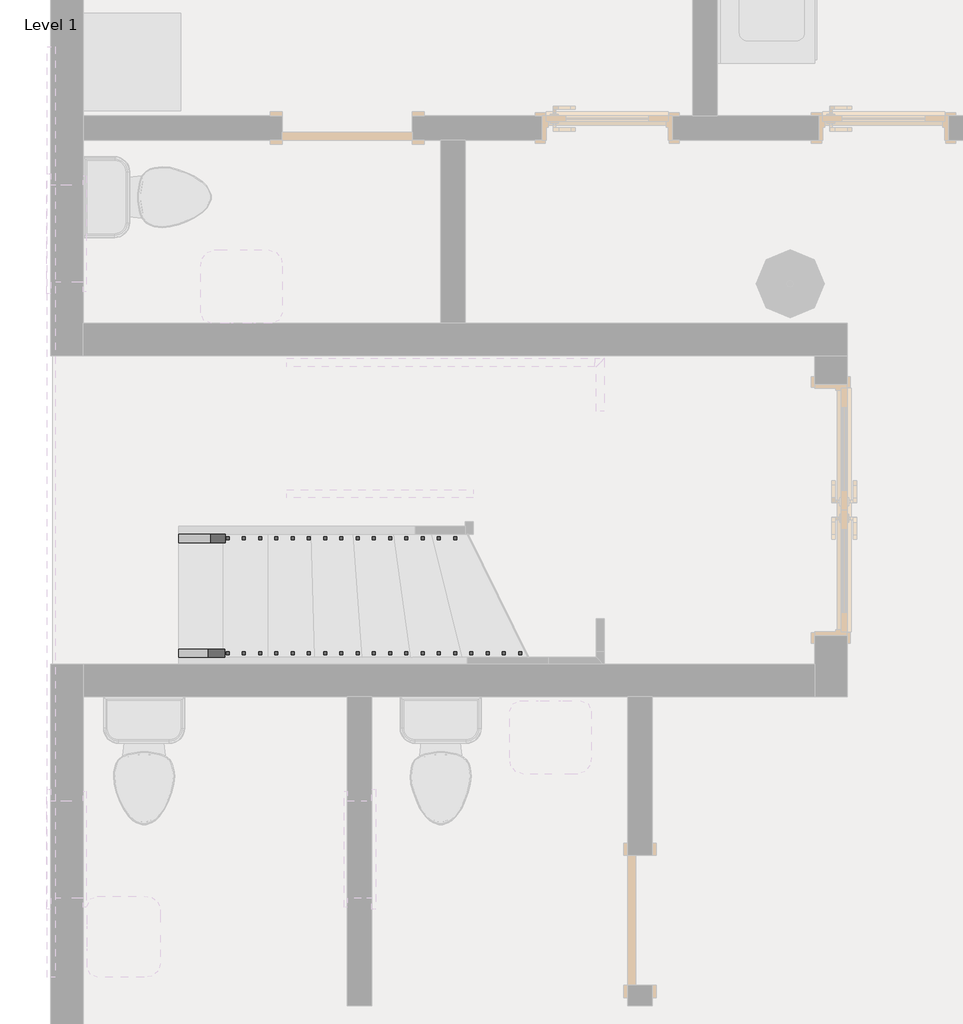
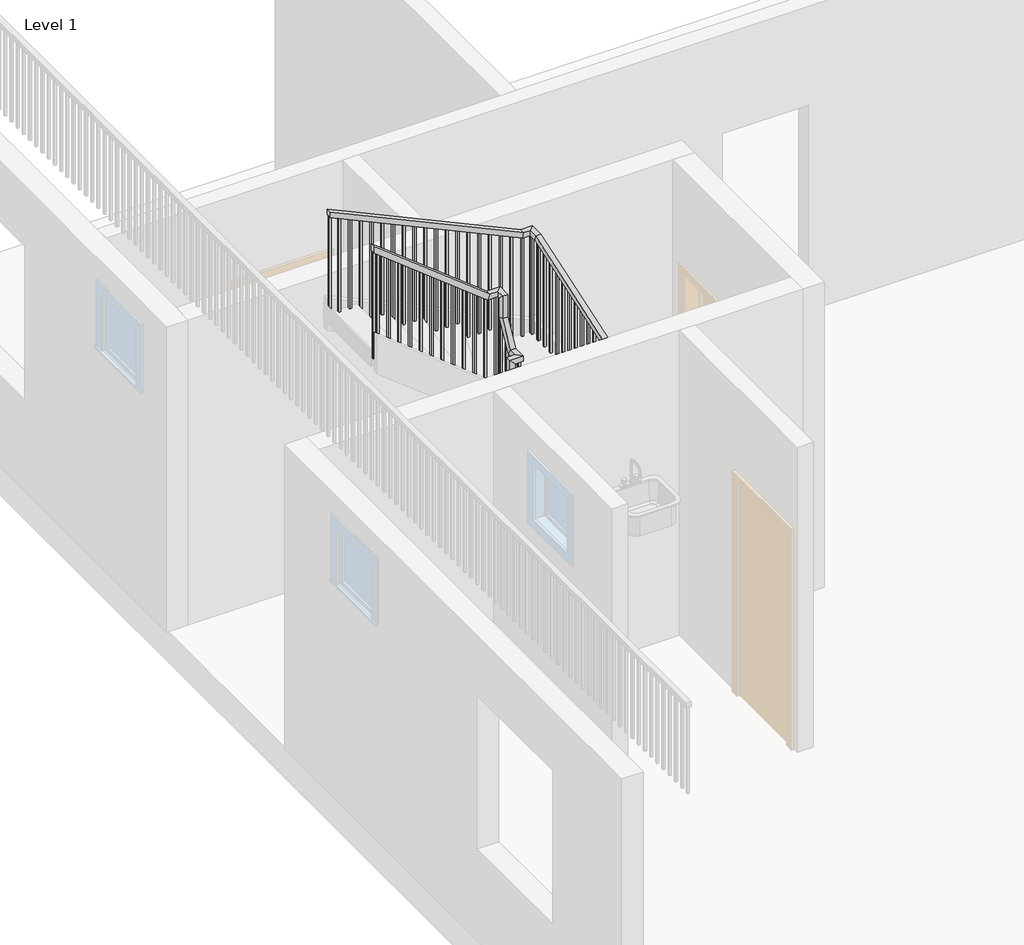
# One storey, part 4 of 7: 2 railings.
"""IFC4 building model written with IfcOpenShell, lengths in millimetres."""

from ifc_helpers import new_model, si_unit, frame, origin, place, context, project, spatial, polyline, outline, extrude, faceted_brep, element, save

model = new_model("IFC4")

# Units and contexts
model_context = context("Model", 3, world=origin())
ifc_project = project(units=[si_unit("LENGTHUNIT", "METRE", prefix="MILLI")], contexts=[model_context])

# Site, building, storey
site = spatial("IfcSite", under=ifc_project)
building = spatial("IfcBuilding", under=site)
storey = spatial("IfcBuildingStorey", under=building, Name="Level 1", Elevation=0.0)

# Railings
placement = place(None, origin())
element("IfcRailing", 1, ObjectType="Handrail - Rectangular", at=placement, inside=storey, context=model_context, shape_type="SolidModel", body=[
    faceted_brep([(-7679.0298583, 5229.7261204, 1101.5391642), (-7679.0298583, 5229.7261204, 1043.7493072), (-7679.0298583, 5178.9261204, 1043.7493072), (-7679.0298583, 5178.9261204, 1101.5391642), (-5235.2838113, 5229.7261204, 2426.8603355), (-5222.395286, 5229.7261204, 2376.0603355), (-5222.395286, 5178.9261204, 2376.0603355), (-5235.2838113, 5178.9261204, 2426.8603355), (-5120.1269231, 5229.7261204, 2376.0603355), (-5120.1269231, 5229.7261204, 2426.8603355), (-5120.1269231, 5429.9022511, 2426.8603355), (-5120.1269231, 5438.2536413, 2376.0603355), (-5069.3269231, 5178.9261204, 2376.0603355), (-5069.3269231, 5438.2536413, 2376.0603355), (-5069.3269231, 5178.9261204, 2426.8603355), (-5069.3269231, 5429.9022511, 2426.8603355), (-5120.1269231, 6946.2417743, 2857.587472), (-5120.1269231, 6946.2417743, 2908.387472), (-5180.0318978, 6946.2417743, 2908.387472), (-5191.2146936, 6946.2417743, 2857.587472), (-5069.3269231, 6997.0417743, 2857.587472), (-5191.2146936, 6997.0417743, 2857.587472), (-5069.3269231, 6997.0417743, 2908.387472), (-5180.0318978, 6997.0417743, 2908.387472), (-5120.1269231, 6854.8426939, 2908.387472), (-5120.1269231, 6863.1940841, 2857.587472), (-5069.3269231, 6863.1940841, 2857.587472), (-5069.3269231, 6854.8426939, 2908.387472), (-7005.4940547, 6946.2417743, 3753.0086233), (-7005.4940547, 6997.0417743, 3753.0086233), (-7005.4940547, 6997.0417743, 3697.0344673), (-7005.4940547, 6946.2417743, 3697.0344673)], [[[0, 1, 2, 3]], [[1, 0, 4, 5]], [[2, 1, 5, 6]], [[3, 2, 6, 7]], [[0, 3, 7, 4]], [[8, 9, 10, 11]], [[12, 8, 11, 13]], [[14, 12, 13, 15]], [[9, 14, 15, 10]], [[16, 17, 18, 19]], [[20, 16, 19, 21]], [[22, 20, 21, 23]], [[17, 22, 23, 18]], [[5, 4, 9, 8]], [[6, 5, 8, 12]], [[7, 6, 12, 14]], [[4, 7, 14, 9]], [[11, 10, 24, 25]], [[13, 11, 25, 26]], [[15, 13, 26, 27]], [[10, 15, 27, 24]], [[25, 24, 17, 16]], [[26, 25, 16, 20]], [[27, 26, 20, 22]], [[24, 27, 22, 17]], [[28, 29, 30, 31]], [[19, 18, 28, 31]], [[21, 19, 31, 30]], [[23, 21, 30, 29]], [[18, 23, 29, 28]]]),
    extrude(outline(polyline([(3647.1625419, -6897.7068978), (3655.9767662, -6916.7568978), (2709.3333333, -6916.7568978), (2709.3333333, -6897.7068978), (3647.1625419, -6897.7068978)])), frame((0.0, 6962.1167743, 0.0), z_axis=(0.0, 1.0, 0.0), x_axis=(0.0, 0.0, 1.0)), (0.0, 0.0, 1.0), 19.05),
    extrude(outline(polyline([(3600.1533456, -6796.1068978), (3608.9675699, -6815.1568978), (2709.3333333, -6815.1568978), (2709.3333333, -6796.1068978), (3600.1533456, -6796.1068978)])), frame((0.0, 6962.1167743, 0.0), z_axis=(0.0, 1.0, 0.0), x_axis=(0.0, 0.0, 1.0)), (0.0, 0.0, 1.0), 19.05),
    extrude(outline(polyline([(3553.1441492, -6694.5068978), (3561.9583735, -6713.5568978), (2540.0, -6713.5568978), (2540.0, -6694.5068978), (3553.1441492, -6694.5068978)])), frame((0.0, 6962.1167743, 0.0), z_axis=(0.0, 1.0, 0.0), x_axis=(0.0, 0.0, 1.0)), (0.0, 0.0, 1.0), 19.05),
    extrude(outline(polyline([(3506.1349529, -6592.9068978), (3514.9491772, -6611.9568978), (2540.0, -6611.9568978), (2540.0, -6592.9068978), (3506.1349529, -6592.9068978)])), frame((0.0, 6962.1167743, 0.0), z_axis=(0.0, 1.0, 0.0), x_axis=(0.0, 0.0, 1.0)), (0.0, 0.0, 1.0), 19.05),
    extrude(outline(polyline([(3459.1257565, -6491.3068978), (3467.9399808, -6510.3568978), (2540.0, -6510.3568978), (2540.0, -6491.3068978), (3459.1257565, -6491.3068978)])), frame((0.0, 6962.1167743, 0.0), z_axis=(0.0, 1.0, 0.0), x_axis=(0.0, 0.0, 1.0)), (0.0, 0.0, 1.0), 19.05),
    extrude(outline(polyline([(3412.1165601, -6389.7068978), (3420.9307845, -6408.7568978), (2370.6666667, -6408.7568978), (2370.6666667, -6389.7068978), (3412.1165601, -6389.7068978)])), frame((0.0, 6962.1167743, 0.0), z_axis=(0.0, 1.0, 0.0), x_axis=(0.0, 0.0, 1.0)), (0.0, 0.0, 1.0), 19.05),
    extrude(outline(polyline([(3365.1073638, -6288.1068978), (3373.9215881, -6307.1568978), (2370.6666667, -6307.1568978), (2370.6666667, -6288.1068978), (3365.1073638, -6288.1068978)])), frame((0.0, 6962.1167743, 0.0), z_axis=(0.0, 1.0, 0.0), x_axis=(0.0, 0.0, 1.0)), (0.0, 0.0, 1.0), 19.05),
    extrude(outline(polyline([(3318.0981674, -6186.5068978), (3326.9123918, -6205.5568978), (2370.6666667, -6205.5568978), (2370.6666667, -6186.5068978), (3318.0981674, -6186.5068978)])), frame((0.0, 6962.1167743, 0.0), z_axis=(0.0, 1.0, 0.0), x_axis=(0.0, 0.0, 1.0)), (0.0, 0.0, 1.0), 19.05),
    extrude(outline(polyline([(3271.0889711, -6084.9068978), (3279.9031954, -6103.9568978), (2201.3333333, -6103.9568978), (2201.3333333, -6084.9068978), (3271.0889711, -6084.9068978)])), frame((0.0, 6962.1167743, 0.0), z_axis=(0.0, 1.0, 0.0), x_axis=(0.0, 0.0, 1.0)), (0.0, 0.0, 1.0), 19.05),
    extrude(outline(polyline([(3224.0797747, -5983.3068978), (3232.8939991, -6002.3568978), (2201.3333333, -6002.3568978), (2201.3333333, -5983.3068978), (3224.0797747, -5983.3068978)])), frame((0.0, 6962.1167743, 0.0), z_axis=(0.0, 1.0, 0.0), x_axis=(0.0, 0.0, 1.0)), (0.0, 0.0, 1.0), 19.05),
    extrude(outline(polyline([(3177.0705784, -5881.7068978), (3185.8848027, -5900.7568978), (2201.3333333, -5900.7568978), (2201.3333333, -5881.7068978), (3177.0705784, -5881.7068978)])), frame((0.0, 6962.1167743, 0.0), z_axis=(0.0, 1.0, 0.0), x_axis=(0.0, 0.0, 1.0)), (0.0, 0.0, 1.0), 19.05),
    extrude(outline(polyline([(3130.061382, -5780.1068978), (3138.8756063, -5799.1568978), (2201.3333333, -5799.1568978), (2201.3333333, -5780.1068978), (3130.061382, -5780.1068978)])), frame((0.0, 6962.1167743, 0.0), z_axis=(0.0, 1.0, 0.0), x_axis=(0.0, 0.0, 1.0)), (0.0, 0.0, 1.0), 19.05),
    extrude(outline(polyline([(3083.0521857, -5678.5068978), (3091.86641, -5697.5568978), (2032.0, -5697.5568978), (2032.0, -5678.5068978), (3083.0521857, -5678.5068978)])), frame((0.0, 6962.1167743, 0.0), z_axis=(0.0, 1.0, 0.0), x_axis=(0.0, 0.0, 1.0)), (0.0, 0.0, 1.0), 19.05),
    extrude(outline(polyline([(3036.0429893, -5576.9068978), (3044.8572136, -5595.9568978), (2032.0, -5595.9568978), (2032.0, -5576.9068978), (3036.0429893, -5576.9068978)])), frame((0.0, 6962.1167743, 0.0), z_axis=(0.0, 1.0, 0.0), x_axis=(0.0, 0.0, 1.0)), (0.0, 0.0, 1.0), 19.05),
    extrude(outline(polyline([(2989.033793, -5475.3068978), (2997.8480173, -5494.3568978), (2032.0, -5494.3568978), (2032.0, -5475.3068978), (2989.033793, -5475.3068978)])), frame((0.0, 6962.1167743, 0.0), z_axis=(0.0, 1.0, 0.0), x_axis=(0.0, 0.0, 1.0)), (0.0, 0.0, 1.0), 19.05),
    extrude(outline(polyline([(2942.0245966, -5373.7068978), (2950.8388209, -5392.7568978), (2032.0, -5392.7568978), (2032.0, -5373.7068978), (2942.0245966, -5373.7068978)])), frame((0.0, 6962.1167743, 0.0), z_axis=(0.0, 1.0, 0.0), x_axis=(0.0, 0.0, 1.0)), (0.0, 0.0, 1.0), 19.05),
    extrude(outline(polyline([(2895.0154003, -5272.1068978), (2903.8296246, -5291.1568978), (1862.6666667, -5291.1568978), (1862.6666667, -5272.1068978), (2895.0154003, -5272.1068978)])), frame((0.0, 6962.1167743, 0.0), z_axis=(0.0, 1.0, 0.0), x_axis=(0.0, 0.0, 1.0)), (0.0, 0.0, 1.0), 19.05),
    extrude(outline(polyline([(-5085.2019231, 6946.9176939), (-5104.2519231, 6946.9176939), (-5104.2519231, 6965.9676939), (-5085.2019231, 6965.9676939), (-5085.2019231, 6946.9176939)])), frame((0.0, 0.0, 1862.6666667), z_axis=(0.0, 0.0, 1.0), x_axis=(1.0, 0.0, 0.0)), (0.0, 0.0, 1.0), 994.9208054),
    extrude(outline(polyline([(6842.7772511, 2850.6880545), (6861.8272511, 2857.125581), (6861.8272511, 1862.6666667), (6842.7772511, 1862.6666667), (6842.7772511, 2850.6880545)])), frame((-5104.2519231, 0.0, 0.0), z_axis=(1.0, 0.0, 0.0), x_axis=(0.0, 1.0, 0.0)), (0.0, 0.0, 1.0), 19.05),
    extrude(outline(polyline([(6741.1772511, 2816.3545795), (6760.2272511, 2822.792106), (6760.2272511, 1862.6666667), (6741.1772511, 1862.6666667), (6741.1772511, 2816.3545795)])), frame((-5104.2519231, 0.0, 0.0), z_axis=(1.0, 0.0, 0.0), x_axis=(0.0, 1.0, 0.0)), (0.0, 0.0, 1.0), 19.05),
    extrude(outline(polyline([(6639.5772511, 2782.0211045), (6658.6272511, 2788.458631), (6658.6272511, 1862.6666667), (6639.5772511, 1862.6666667), (6639.5772511, 2782.0211045)])), frame((-5104.2519231, 0.0, 0.0), z_axis=(1.0, 0.0, 0.0), x_axis=(0.0, 1.0, 0.0)), (0.0, 0.0, 1.0), 19.05),
    extrude(outline(polyline([(6537.9772511, 2747.6876295), (6557.0272511, 2754.125156), (6557.0272511, 1862.6666667), (6537.9772511, 1862.6666667), (6537.9772511, 2747.6876295)])), frame((-5104.2519231, 0.0, 0.0), z_axis=(1.0, 0.0, 0.0), x_axis=(0.0, 1.0, 0.0)), (0.0, 0.0, 1.0), 19.05),
    extrude(outline(polyline([(6436.3772511, 2713.3541545), (6455.4272511, 2719.791681), (6455.4272511, 1693.3333333), (6436.3772511, 1693.3333333), (6436.3772511, 2713.3541545)])), frame((-5104.2519231, 0.0, 0.0), z_axis=(1.0, 0.0, 0.0), x_axis=(0.0, 1.0, 0.0)), (0.0, 0.0, 1.0), 19.05),
    extrude(outline(polyline([(6334.7772511, 2679.0206795), (6353.8272511, 2685.458206), (6353.8272511, 1693.3333333), (6334.7772511, 1693.3333333), (6334.7772511, 2679.0206795)])), frame((-5104.2519231, 0.0, 0.0), z_axis=(1.0, 0.0, 0.0), x_axis=(0.0, 1.0, 0.0)), (0.0, 0.0, 1.0), 19.05),
    extrude(outline(polyline([(6233.1772511, 2644.6872045), (6252.2272511, 2651.124731), (6252.2272511, 1693.3333333), (6233.1772511, 1693.3333333), (6233.1772511, 2644.6872045)])), frame((-5104.2519231, 0.0, 0.0), z_axis=(1.0, 0.0, 0.0), x_axis=(0.0, 1.0, 0.0)), (0.0, 0.0, 1.0), 19.05),
    extrude(outline(polyline([(6131.5772511, 2610.3537294), (6150.6272511, 2616.791256), (6150.6272511, 1693.3333333), (6131.5772511, 1693.3333333), (6131.5772511, 2610.3537294)])), frame((-5104.2519231, 0.0, 0.0), z_axis=(1.0, 0.0, 0.0), x_axis=(0.0, 1.0, 0.0)), (0.0, 0.0, 1.0), 19.05),
    extrude(outline(polyline([(6029.9772511, 2576.0202544), (6049.0272511, 2582.457781), (6049.0272511, 1693.3333333), (6029.9772511, 1693.3333333), (6029.9772511, 2576.0202544)])), frame((-5104.2519231, 0.0, 0.0), z_axis=(1.0, 0.0, 0.0), x_axis=(0.0, 1.0, 0.0)), (0.0, 0.0, 1.0), 19.05),
    extrude(outline(polyline([(5928.3772511, 2541.6867794), (5947.4272511, 2548.124306), (5947.4272511, 1524.0), (5928.3772511, 1524.0), (5928.3772511, 2541.6867794)])), frame((-5104.2519231, 0.0, 0.0), z_axis=(1.0, 0.0, 0.0), x_axis=(0.0, 1.0, 0.0)), (0.0, 0.0, 1.0), 19.05),
    extrude(outline(polyline([(5826.7772511, 2507.3533044), (5845.8272511, 2513.790831), (5845.8272511, 1524.0), (5826.7772511, 1524.0), (5826.7772511, 2507.3533044)])), frame((-5104.2519231, 0.0, 0.0), z_axis=(1.0, 0.0, 0.0), x_axis=(0.0, 1.0, 0.0)), (0.0, 0.0, 1.0), 19.05),
    extrude(outline(polyline([(5725.1772511, 2473.0198294), (5744.2272511, 2479.457356), (5744.2272511, 1524.0), (5725.1772511, 1524.0), (5725.1772511, 2473.0198294)])), frame((-5104.2519231, 0.0, 0.0), z_axis=(1.0, 0.0, 0.0), x_axis=(0.0, 1.0, 0.0)), (0.0, 0.0, 1.0), 19.05),
    extrude(outline(polyline([(5623.5772511, 2438.6863544), (5642.6272511, 2445.123881), (5642.6272511, 1524.0), (5623.5772511, 1524.0), (5623.5772511, 2438.6863544)])), frame((-5104.2519231, 0.0, 0.0), z_axis=(1.0, 0.0, 0.0), x_axis=(0.0, 1.0, 0.0)), (0.0, 0.0, 1.0), 19.05),
    extrude(outline(polyline([(5521.9772511, 2404.3528794), (5541.0272511, 2410.790406), (5541.0272511, 1524.0), (5521.9772511, 1524.0), (5521.9772511, 2404.3528794)])), frame((-5104.2519231, 0.0, 0.0), z_axis=(1.0, 0.0, 0.0), x_axis=(0.0, 1.0, 0.0)), (0.0, 0.0, 1.0), 19.05),
    extrude(outline(polyline([(-5085.2019231, 5398.0011204), (-5104.2519231, 5398.0011204), (-5104.2519231, 5417.0511204), (-5085.2019231, 5417.0511204), (-5085.2019231, 5398.0011204)])), frame((0.0, 0.0, 1354.6666667), z_axis=(0.0, 0.0, 1.0), x_axis=(1.0, 0.0, 0.0)), (0.0, 0.0, 1.0), 1021.3936688),
    extrude(outline(polyline([(-5085.2019231, 5296.4011204), (-5104.2519231, 5296.4011204), (-5104.2519231, 5315.4511204), (-5085.2019231, 5315.4511204), (-5085.2019231, 5296.4011204)])), frame((0.0, 0.0, 1354.6666667), z_axis=(0.0, 0.0, 1.0), x_axis=(1.0, 0.0, 0.0)), (0.0, 0.0, 1.0), 1021.3936688),
    extrude(outline(polyline([(-5143.2088113, 5194.8011204), (-5143.2088113, 5213.8511204), (-5124.1588113, 5213.8511204), (-5124.1588113, 5194.8011204), (-5143.2088113, 5194.8011204)])), frame((0.0, 0.0, 1354.6666667), z_axis=(0.0, 0.0, 1.0), x_axis=(1.0, 0.0, 0.0)), (0.0, 0.0, 1.0), 1021.3936688),
    extrude(outline(polyline([(2371.3368575, -5231.1048583), (2361.0054369, -5250.1548583), (1354.6666667, -5250.1548583), (1354.6666667, -5231.1048583), (2371.3368575, -5231.1048583)])), frame((0.0, 5194.8011204, 0.0), z_axis=(0.0, 1.0, 0.0), x_axis=(0.0, 0.0, 1.0)), (0.0, 0.0, 1.0), 19.05),
    extrude(outline(polyline([(2316.2359475, -5332.7048583), (2305.9045269, -5351.7548583), (1354.6666667, -5351.7548583), (1354.6666667, -5332.7048583), (2316.2359475, -5332.7048583)])), frame((0.0, 5194.8011204, 0.0), z_axis=(0.0, 1.0, 0.0), x_axis=(0.0, 0.0, 1.0)), (0.0, 0.0, 1.0), 19.05),
    extrude(outline(polyline([(2261.1350375, -5434.3048583), (2250.8036169, -5453.3548583), (1354.6666667, -5453.3548583), (1354.6666667, -5434.3048583), (2261.1350375, -5434.3048583)])), frame((0.0, 5194.8011204, 0.0), z_axis=(0.0, 1.0, 0.0), x_axis=(0.0, 0.0, 1.0)), (0.0, 0.0, 1.0), 19.05),
    extrude(outline(polyline([(2206.0341275, -5535.9048583), (2195.7027069, -5554.9548583), (1185.3333333, -5554.9548583), (1185.3333333, -5535.9048583), (2206.0341275, -5535.9048583)])), frame((0.0, 5194.8011204, 0.0), z_axis=(0.0, 1.0, 0.0), x_axis=(0.0, 0.0, 1.0)), (0.0, 0.0, 1.0), 19.05),
    extrude(outline(polyline([(2150.9332175, -5637.5048583), (2140.6017969, -5656.5548583), (1185.3333333, -5656.5548583), (1185.3333333, -5637.5048583), (2150.9332175, -5637.5048583)])), frame((0.0, 5194.8011204, 0.0), z_axis=(0.0, 1.0, 0.0), x_axis=(0.0, 0.0, 1.0)), (0.0, 0.0, 1.0), 19.05),
    extrude(outline(polyline([(2095.8323075, -5739.1048583), (2085.5008869, -5758.1548583), (1185.3333333, -5758.1548583), (1185.3333333, -5739.1048583), (2095.8323075, -5739.1048583)])), frame((0.0, 5194.8011204, 0.0), z_axis=(0.0, 1.0, 0.0), x_axis=(0.0, 0.0, 1.0)), (0.0, 0.0, 1.0), 19.05),
    extrude(outline(polyline([(2040.7313975, -5840.7048583), (2030.3999769, -5859.7548583), (1185.3333333, -5859.7548583), (1185.3333333, -5840.7048583), (2040.7313975, -5840.7048583)])), frame((0.0, 5194.8011204, 0.0), z_axis=(0.0, 1.0, 0.0), x_axis=(0.0, 0.0, 1.0)), (0.0, 0.0, 1.0), 19.05),
    extrude(outline(polyline([(1985.6304875, -5942.3048583), (1975.2990669, -5961.3548583), (1016.0, -5961.3548583), (1016.0, -5942.3048583), (1985.6304875, -5942.3048583)])), frame((0.0, 5194.8011204, 0.0), z_axis=(0.0, 1.0, 0.0), x_axis=(0.0, 0.0, 1.0)), (0.0, 0.0, 1.0), 19.05),
    extrude(outline(polyline([(1930.5295775, -6043.9048583), (1920.1981569, -6062.9548583), (1016.0, -6062.9548583), (1016.0, -6043.9048583), (1930.5295775, -6043.9048583)])), frame((0.0, 5194.8011204, 0.0), z_axis=(0.0, 1.0, 0.0), x_axis=(0.0, 0.0, 1.0)), (0.0, 0.0, 1.0), 19.05),
    extrude(outline(polyline([(1875.4286675, -6145.5048583), (1865.0972469, -6164.5548583), (1016.0, -6164.5548583), (1016.0, -6145.5048583), (1875.4286675, -6145.5048583)])), frame((0.0, 5194.8011204, 0.0), z_axis=(0.0, 1.0, 0.0), x_axis=(0.0, 0.0, 1.0)), (0.0, 0.0, 1.0), 19.05),
    extrude(outline(polyline([(1820.3277575, -6247.1048583), (1809.9963369, -6266.1548583), (846.6666667, -6266.1548583), (846.6666667, -6247.1048583), (1820.3277575, -6247.1048583)])), frame((0.0, 5194.8011204, 0.0), z_axis=(0.0, 1.0, 0.0), x_axis=(0.0, 0.0, 1.0)), (0.0, 0.0, 1.0), 19.05),
    extrude(outline(polyline([(1765.2268475, -6348.7048583), (1754.8954269, -6367.7548583), (846.6666667, -6367.7548583), (846.6666667, -6348.7048583), (1765.2268475, -6348.7048583)])), frame((0.0, 5194.8011204, 0.0), z_axis=(0.0, 1.0, 0.0), x_axis=(0.0, 0.0, 1.0)), (0.0, 0.0, 1.0), 19.05),
    extrude(outline(polyline([(1710.1259375, -6450.3048583), (1699.7945169, -6469.3548583), (846.6666667, -6469.3548583), (846.6666667, -6450.3048583), (1710.1259375, -6450.3048583)])), frame((0.0, 5194.8011204, 0.0), z_axis=(0.0, 1.0, 0.0), x_axis=(0.0, 0.0, 1.0)), (0.0, 0.0, 1.0), 19.05),
    extrude(outline(polyline([(1655.0250275, -6551.9048583), (1644.6936069, -6570.9548583), (677.3333333, -6570.9548583), (677.3333333, -6551.9048583), (1655.0250275, -6551.9048583)])), frame((0.0, 5194.8011204, 0.0), z_axis=(0.0, 1.0, 0.0), x_axis=(0.0, 0.0, 1.0)), (0.0, 0.0, 1.0), 19.05),
    extrude(outline(polyline([(1599.9241175, -6653.5048583), (1589.5926969, -6672.5548583), (677.3333333, -6672.5548583), (677.3333333, -6653.5048583), (1599.9241175, -6653.5048583)])), frame((0.0, 5194.8011204, 0.0), z_axis=(0.0, 1.0, 0.0), x_axis=(0.0, 0.0, 1.0)), (0.0, 0.0, 1.0), 19.05),
    extrude(outline(polyline([(1544.8232075, -6755.1048583), (1534.4917869, -6774.1548583), (677.3333333, -6774.1548583), (677.3333333, -6755.1048583), (1544.8232075, -6755.1048583)])), frame((0.0, 5194.8011204, 0.0), z_axis=(0.0, 1.0, 0.0), x_axis=(0.0, 0.0, 1.0)), (0.0, 0.0, 1.0), 19.05),
    extrude(outline(polyline([(1489.7222975, -6856.7048583), (1479.3908769, -6875.7548583), (508.0, -6875.7548583), (508.0, -6856.7048583), (1489.7222975, -6856.7048583)])), frame((0.0, 5194.8011204, 0.0), z_axis=(0.0, 1.0, 0.0), x_axis=(0.0, 0.0, 1.0)), (0.0, 0.0, 1.0), 19.05),
    extrude(outline(polyline([(1434.6213875, -6958.3048583), (1424.2899669, -6977.3548583), (508.0, -6977.3548583), (508.0, -6958.3048583), (1434.6213875, -6958.3048583)])), frame((0.0, 5194.8011204, 0.0), z_axis=(0.0, 1.0, 0.0), x_axis=(0.0, 0.0, 1.0)), (0.0, 0.0, 1.0), 19.05),
    extrude(outline(polyline([(1379.5204775, -7059.9048583), (1369.1890569, -7078.9548583), (508.0, -7078.9548583), (508.0, -7059.9048583), (1379.5204775, -7059.9048583)])), frame((0.0, 5194.8011204, 0.0), z_axis=(0.0, 1.0, 0.0), x_axis=(0.0, 0.0, 1.0)), (0.0, 0.0, 1.0), 19.05),
    extrude(outline(polyline([(1324.4195675, -7161.5048583), (1314.0881469, -7180.5548583), (338.6666667, -7180.5548583), (338.6666667, -7161.5048583), (1324.4195675, -7161.5048583)])), frame((0.0, 5194.8011204, 0.0), z_axis=(0.0, 1.0, 0.0), x_axis=(0.0, 0.0, 1.0)), (0.0, 0.0, 1.0), 19.05),
    extrude(outline(polyline([(1269.3186575, -7263.1048583), (1258.9872369, -7282.1548583), (338.6666667, -7282.1548583), (338.6666667, -7263.1048583), (1269.3186575, -7263.1048583)])), frame((0.0, 5194.8011204, 0.0), z_axis=(0.0, 1.0, 0.0), x_axis=(0.0, 0.0, 1.0)), (0.0, 0.0, 1.0), 19.05),
    extrude(outline(polyline([(1214.2177475, -7364.7048583), (1203.8863269, -7383.7548583), (338.6666667, -7383.7548583), (338.6666667, -7364.7048583), (1214.2177475, -7364.7048583)])), frame((0.0, 5194.8011204, 0.0), z_axis=(0.0, 1.0, 0.0), x_axis=(0.0, 0.0, 1.0)), (0.0, 0.0, 1.0), 19.05),
    extrude(outline(polyline([(1159.1168375, -7466.3048583), (1148.7854169, -7485.3548583), (169.3333333, -7485.3548583), (169.3333333, -7466.3048583), (1159.1168375, -7466.3048583)])), frame((0.0, 5194.8011204, 0.0), z_axis=(0.0, 1.0, 0.0), x_axis=(0.0, 0.0, 1.0)), (0.0, 0.0, 1.0), 19.05),
    extrude(outline(polyline([(1104.0159275, -7567.9048583), (1093.6845069, -7586.9548583), (169.3333333, -7586.9548583), (169.3333333, -7567.9048583), (1104.0159275, -7567.9048583)])), frame((0.0, 5194.8011204, 0.0), z_axis=(0.0, 1.0, 0.0), x_axis=(0.0, 0.0, 1.0)), (0.0, 0.0, 1.0), 19.05),
    extrude(outline(polyline([(-5170.5068978, 6981.1667743), (-5170.5068978, 6962.1167743), (-5189.5568978, 6962.1167743), (-5189.5568978, 6981.1667743), (-5170.5068978, 6981.1667743)])), frame((0.0, 0.0, 1862.6666667), z_axis=(0.0, 0.0, 1.0), x_axis=(1.0, 0.0, 0.0)), (0.0, 0.0, 1.0), 994.9208054),
    extrude(outline(polyline([(-5085.2019231, 6962.1167743), (-5104.2519231, 6962.1167743), (-5104.2519231, 6981.1667743), (-5085.2019231, 6981.1667743), (-5085.2019231, 6962.1167743)])), frame((0.0, 0.0, 1862.6666667), z_axis=(0.0, 0.0, 1.0), x_axis=(1.0, 0.0, 0.0)), (0.0, 0.0, 1.0), 994.9208054),
    extrude(outline(polyline([(6845.3176939, 2851.546541), (6864.3676939, 2857.9840675), (6864.3676939, 1862.6666667), (6845.3176939, 1862.6666667), (6845.3176939, 2851.546541)])), frame((-5104.2519231, 0.0, 0.0), z_axis=(1.0, 0.0, 0.0), x_axis=(0.0, 1.0, 0.0)), (0.0, 0.0, 1.0), 19.05),
    extrude(outline(polyline([(-5085.2019231, 5420.3772511), (-5104.2519231, 5420.3772511), (-5104.2519231, 5439.4272511), (-5085.2019231, 5439.4272511), (-5085.2019231, 5420.3772511)])), frame((0.0, 0.0, 1354.6666667), z_axis=(0.0, 0.0, 1.0), x_axis=(1.0, 0.0, 0.0)), (0.0, 0.0, 1.0), 1021.3936688),
    extrude(outline(polyline([(-5104.2519231, 5194.8011204), (-5104.2519231, 5213.8511204), (-5085.2019231, 5213.8511204), (-5085.2019231, 5194.8011204), (-5104.2519231, 5194.8011204)])), frame((0.0, 0.0, 1354.6666667), z_axis=(0.0, 0.0, 1.0), x_axis=(1.0, 0.0, 0.0)), (0.0, 0.0, 1.0), 1021.3936688),
    extrude(outline(polyline([(2374.2361888, -5225.7588113), (2363.9047682, -5244.8088113), (1354.6666667, -5244.8088113), (1354.6666667, -5225.7588113), (2374.2361888, -5225.7588113)])), frame((0.0, 5194.8011204, 0.0), z_axis=(0.0, 1.0, 0.0), x_axis=(0.0, 0.0, 1.0)), (0.0, 0.0, 1.0), 19.05),
    extrude(outline(polyline([(3688.220243, -6986.4440547), (3697.0344673, -7005.4940547), (2709.3333333, -7005.4940547), (2709.3333333, -6986.4440547), (3688.220243, -6986.4440547)])), frame((0.0, 6962.1167743, 0.0), z_axis=(0.0, 1.0, 0.0), x_axis=(0.0, 0.0, 1.0)), (0.0, 0.0, 1.0), 19.05),
    extrude(outline(polyline([(1054.0807278, -7659.9798583), (1043.7493072, -7679.0298583), (169.3333333, -7679.0298583), (169.3333333, -7659.9798583), (1054.0807278, -7659.9798583)])), frame((0.0, 5194.8011204, 0.0), z_axis=(0.0, 1.0, 0.0), x_axis=(0.0, 0.0, 1.0)), (0.0, 0.0, 1.0), 19.05),
])
element("IfcRailing", 2, ObjectType="Handrail - Rectangular", at=placement, inside=storey, context=model_context, shape_type="SolidModel", body=[
    faceted_brep([(-7679.0298583, 5948.2839473, 1063.2569244), (-7679.0298583, 5948.2839473, 1001.8432483), (-7679.0298583, 5897.4839473, 1001.8432483), (-7679.0298583, 5897.4839473, 1063.2569244), (-5914.88475, 5948.2839473, 2261.724814), (-5864.08475, 5948.2839473, 2234.8220001), (-5864.08475, 5897.4839473, 2234.8220001), (-5914.88475, 5897.4839473, 2261.724814), (-5838.68475, 6054.8875761, 2473.5239648), (-5838.68475, 6024.4839473, 2524.3239648), (-5838.68475, 6151.4839473, 2761.1854815), (-5838.68475, 6202.2839473, 2748.4257604), (-5787.88475, 6054.8875761, 2473.5239648), (-5787.88475, 6202.2839473, 2748.4257604), (-5787.88475, 6024.4839473, 2524.3239648), (-5787.88475, 6151.4839473, 2761.1854815), (-7005.4940547, 6227.6839473, 3843.0590007), (-7005.4940547, 6278.4839473, 3843.0590007), (-7005.4940547, 6278.4839473, 3778.4769091), (-7005.4940547, 6227.6839473, 3778.4769091), (-5932.4418214, 6227.6839473, 2936.143705), (-5914.88475, 6227.6839473, 2986.943705), (-5932.4418214, 6278.4839473, 2936.143705), (-5914.88475, 6278.4839473, 2986.943705), (-5914.88475, 5948.2839473, 2524.3239648), (-5864.08475, 5948.2839473, 2473.5239648), (-5864.08475, 5897.4839473, 2473.5239648), (-5914.88475, 5897.4839473, 2524.3239648), (-5838.68475, 5948.2839473, 2524.3239648), (-5838.68475, 5948.2839473, 2473.5239648), (-5787.88475, 5897.4839473, 2473.5239648), (-5787.88475, 5897.4839473, 2524.3239648), (-5838.68475, 6151.4839473, 2986.943705), (-5838.68475, 6202.2839473, 2936.143705), (-5787.88475, 6202.2839473, 2936.143705), (-5787.88475, 6151.4839473, 2986.943705), (-5838.68475, 6227.6839473, 2986.943705), (-5838.68475, 6227.6839473, 2936.143705), (-5787.88475, 6278.4839473, 2936.143705), (-5787.88475, 6278.4839473, 2986.943705)], [[[0, 1, 2, 3]], [[1, 0, 4, 5]], [[2, 1, 5, 6]], [[3, 2, 6, 7]], [[0, 3, 7, 4]], [[8, 9, 10, 11]], [[12, 8, 11, 13]], [[14, 12, 13, 15]], [[9, 14, 15, 10]], [[16, 17, 18, 19]], [[20, 21, 16, 19]], [[22, 20, 19, 18]], [[23, 22, 18, 17]], [[21, 23, 17, 16]], [[5, 4, 24, 25]], [[6, 5, 25, 26]], [[7, 6, 26, 27]], [[4, 7, 27, 24]], [[25, 24, 28, 29]], [[26, 25, 29, 30]], [[27, 26, 30, 31]], [[24, 27, 31, 28]], [[29, 28, 9, 8]], [[30, 29, 8, 12]], [[31, 30, 12, 14]], [[28, 31, 14, 9]], [[11, 10, 32, 33]], [[13, 11, 33, 34]], [[15, 13, 34, 35]], [[10, 15, 35, 32]], [[33, 32, 36, 37]], [[34, 33, 37, 38]], [[35, 34, 38, 39]], [[32, 35, 39, 36]], [[37, 36, 21, 20]], [[38, 37, 20, 22]], [[39, 38, 22, 23]], [[36, 39, 23, 21]]]),
    extrude(outline(polyline([(3749.1293953, -6968.1081187), (2709.3333333, -6968.1081187), (2709.3333333, -6949.0581187), (3734.1753725, -6949.0581187), (3749.1293953, -6968.1081187)])), frame((0.0, 6243.5589473, 0.0), z_axis=(0.0, 1.0, 0.0), x_axis=(0.0, 0.0, 1.0)), (0.0, 0.0, 1.0), 19.05),
    extrude(outline(polyline([(3669.3746071, -6866.5081187), (2709.3333333, -6866.5081187), (2709.3333333, -6847.4581187), (3654.4205844, -6847.4581187), (3669.3746071, -6866.5081187)])), frame((0.0, 6243.5589473, 0.0), z_axis=(0.0, 1.0, 0.0), x_axis=(0.0, 0.0, 1.0)), (0.0, 0.0, 1.0), 19.05),
    extrude(outline(polyline([(3589.619819, -6764.9081187), (2709.3333333, -6764.9081187), (2709.3333333, -6745.8581187), (3574.6657962, -6745.8581187), (3589.619819, -6764.9081187)])), frame((0.0, 6243.5589473, 0.0), z_axis=(0.0, 1.0, 0.0), x_axis=(0.0, 0.0, 1.0)), (0.0, 0.0, 1.0), 19.05),
    extrude(outline(polyline([(3509.8650309, -6663.3081187), (2540.0, -6663.3081187), (2540.0, -6644.2581187), (3494.9110081, -6644.2581187), (3509.8650309, -6663.3081187)])), frame((0.0, 6243.5589473, 0.0), z_axis=(0.0, 1.0, 0.0), x_axis=(0.0, 0.0, 1.0)), (0.0, 0.0, 1.0), 19.05),
    extrude(outline(polyline([(3430.1102427, -6561.7081187), (2540.0, -6561.7081187), (2540.0, -6542.6581187), (3415.1562199, -6542.6581187), (3430.1102427, -6561.7081187)])), frame((0.0, 6243.5589473, 0.0), z_axis=(0.0, 1.0, 0.0), x_axis=(0.0, 0.0, 1.0)), (0.0, 0.0, 1.0), 19.05),
    extrude(outline(polyline([(3350.3554546, -6460.1081187), (2540.0, -6460.1081187), (2540.0, -6441.0581187), (3335.4014318, -6441.0581187), (3350.3554546, -6460.1081187)])), frame((0.0, 6243.5589473, 0.0), z_axis=(0.0, 1.0, 0.0), x_axis=(0.0, 0.0, 1.0)), (0.0, 0.0, 1.0), 19.05),
    extrude(outline(polyline([(3270.6006664, -6358.5081187), (2370.6666667, -6358.5081187), (2370.6666667, -6339.4581187), (3255.6466436, -6339.4581187), (3270.6006664, -6358.5081187)])), frame((0.0, 6243.5589473, 0.0), z_axis=(0.0, 1.0, 0.0), x_axis=(0.0, 0.0, 1.0)), (0.0, 0.0, 1.0), 19.05),
    extrude(outline(polyline([(3190.8458783, -6256.9081187), (2370.6666667, -6256.9081187), (2370.6666667, -6237.8581187), (3175.8918555, -6237.8581187), (3190.8458783, -6256.9081187)])), frame((0.0, 6243.5589473, 0.0), z_axis=(0.0, 1.0, 0.0), x_axis=(0.0, 0.0, 1.0)), (0.0, 0.0, 1.0), 19.05),
    extrude(outline(polyline([(3111.0910901, -6155.3081187), (2201.3333333, -6155.3081187), (2201.3333333, -6136.2581187), (3096.1370673, -6136.2581187), (3111.0910901, -6155.3081187)])), frame((0.0, 6243.5589473, 0.0), z_axis=(0.0, 1.0, 0.0), x_axis=(0.0, 0.0, 1.0)), (0.0, 0.0, 1.0), 19.05),
    extrude(outline(polyline([(3031.336302, -6053.7081187), (2201.3333333, -6053.7081187), (2201.3333333, -6034.6581187), (3016.3822792, -6034.6581187), (3031.336302, -6053.7081187)])), frame((0.0, 6243.5589473, 0.0), z_axis=(0.0, 1.0, 0.0), x_axis=(0.0, 0.0, 1.0)), (0.0, 0.0, 1.0), 19.05),
    extrude(outline(polyline([(2951.5815138, -5952.1081187), (2032.0, -5952.1081187), (2032.0, -5933.0581187), (2936.627491, -5933.0581187), (2951.5815138, -5952.1081187)])), frame((0.0, 6243.5589473, 0.0), z_axis=(0.0, 1.0, 0.0), x_axis=(0.0, 0.0, 1.0)), (0.0, 0.0, 1.0), 19.05),
    extrude(outline(polyline([(-5822.80975, 6218.1589473), (-5822.80975, 6237.2089473), (-5803.75975, 6237.2089473), (-5803.75975, 6218.1589473), (-5822.80975, 6218.1589473)])), frame((0.0, 0.0, 1862.6666667), z_axis=(0.0, 0.0, 1.0), x_axis=(1.0, 0.0, 0.0)), (0.0, 0.0, 1.0), 1073.4770384),
    extrude(outline(polyline([(6135.6089473, 2624.0734642), (6135.6089473, 1693.3333333), (6116.5589473, 1693.3333333), (6116.5589473, 2588.5442366), (6135.6089473, 2624.0734642)])), frame((-5822.80975, 0.0, 0.0), z_axis=(1.0, 0.0, 0.0), x_axis=(0.0, 1.0, 0.0)), (0.0, 0.0, 1.0), 19.05),
    extrude(outline(polyline([(-5822.80975, 6014.9589473), (-5822.80975, 6034.0089473), (-5803.75975, 6034.0089473), (-5803.75975, 6014.9589473), (-5822.80975, 6014.9589473)])), frame((0.0, 0.0, 1524.0), z_axis=(0.0, 0.0, 1.0), x_axis=(1.0, 0.0, 0.0)), (0.0, 0.0, 1.0), 949.5239648),
    extrude(outline(polyline([(-5859.7548583, 5932.4089473), (-5840.7048583, 5932.4089473), (-5840.7048583, 5913.3589473), (-5859.7548583, 5913.3589473), (-5859.7548583, 5932.4089473)])), frame((0.0, 0.0, 1354.6666667), z_axis=(0.0, 0.0, 1.0), x_axis=(1.0, 0.0, 0.0)), (0.0, 0.0, 1.0), 1118.8572982),
    extrude(outline(polyline([(2168.7417775, -5961.3548583), (1185.3333333, -5961.3548583), (1185.3333333, -5942.3048583), (2181.6833509, -5942.3048583), (2168.7417775, -5961.3548583)])), frame((0.0, 5913.3589473, 0.0), z_axis=(0.0, 1.0, 0.0), x_axis=(0.0, 0.0, 1.0)), (0.0, 0.0, 1.0), 19.05),
    extrude(outline(polyline([(2099.7200531, -6062.9548583), (1185.3333333, -6062.9548583), (1185.3333333, -6043.9048583), (2112.6616264, -6043.9048583), (2099.7200531, -6062.9548583)])), frame((0.0, 5913.3589473, 0.0), z_axis=(0.0, 1.0, 0.0), x_axis=(0.0, 0.0, 1.0)), (0.0, 0.0, 1.0), 19.05),
    extrude(outline(polyline([(2030.6983286, -6164.5548583), (1016.0, -6164.5548583), (1016.0, -6145.5048583), (2043.6399019, -6145.5048583), (2030.6983286, -6164.5548583)])), frame((0.0, 5913.3589473, 0.0), z_axis=(0.0, 1.0, 0.0), x_axis=(0.0, 0.0, 1.0)), (0.0, 0.0, 1.0), 19.05),
    extrude(outline(polyline([(1961.6766041, -6266.1548583), (1016.0, -6266.1548583), (1016.0, -6247.1048583), (1974.6181775, -6247.1048583), (1961.6766041, -6266.1548583)])), frame((0.0, 5913.3589473, 0.0), z_axis=(0.0, 1.0, 0.0), x_axis=(0.0, 0.0, 1.0)), (0.0, 0.0, 1.0), 19.05),
    extrude(outline(polyline([(1892.6548797, -6367.7548583), (846.6666667, -6367.7548583), (846.6666667, -6348.7048583), (1905.596453, -6348.7048583), (1892.6548797, -6367.7548583)])), frame((0.0, 5913.3589473, 0.0), z_axis=(0.0, 1.0, 0.0), x_axis=(0.0, 0.0, 1.0)), (0.0, 0.0, 1.0), 19.05),
    extrude(outline(polyline([(1823.6331552, -6469.3548583), (846.6666667, -6469.3548583), (846.6666667, -6450.3048583), (1836.5747285, -6450.3048583), (1823.6331552, -6469.3548583)])), frame((0.0, 5913.3589473, 0.0), z_axis=(0.0, 1.0, 0.0), x_axis=(0.0, 0.0, 1.0)), (0.0, 0.0, 1.0), 19.05),
    extrude(outline(polyline([(1754.6114307, -6570.9548583), (846.6666667, -6570.9548583), (846.6666667, -6551.9048583), (1767.5530041, -6551.9048583), (1754.6114307, -6570.9548583)])), frame((0.0, 5913.3589473, 0.0), z_axis=(0.0, 1.0, 0.0), x_axis=(0.0, 0.0, 1.0)), (0.0, 0.0, 1.0), 19.05),
    extrude(outline(polyline([(1685.5897063, -6672.5548583), (677.3333333, -6672.5548583), (677.3333333, -6653.5048583), (1698.5312796, -6653.5048583), (1685.5897063, -6672.5548583)])), frame((0.0, 5913.3589473, 0.0), z_axis=(0.0, 1.0, 0.0), x_axis=(0.0, 0.0, 1.0)), (0.0, 0.0, 1.0), 19.05),
    extrude(outline(polyline([(1616.5679818, -6774.1548583), (677.3333333, -6774.1548583), (677.3333333, -6755.1048583), (1629.5095551, -6755.1048583), (1616.5679818, -6774.1548583)])), frame((0.0, 5913.3589473, 0.0), z_axis=(0.0, 1.0, 0.0), x_axis=(0.0, 0.0, 1.0)), (0.0, 0.0, 1.0), 19.05),
    extrude(outline(polyline([(1547.5462573, -6875.7548583), (508.0, -6875.7548583), (508.0, -6856.7048583), (1560.4878307, -6856.7048583), (1547.5462573, -6875.7548583)])), frame((0.0, 5913.3589473, 0.0), z_axis=(0.0, 1.0, 0.0), x_axis=(0.0, 0.0, 1.0)), (0.0, 0.0, 1.0), 19.05),
    extrude(outline(polyline([(1478.5245329, -6977.3548583), (508.0, -6977.3548583), (508.0, -6958.3048583), (1491.4661062, -6958.3048583), (1478.5245329, -6977.3548583)])), frame((0.0, 5913.3589473, 0.0), z_axis=(0.0, 1.0, 0.0), x_axis=(0.0, 0.0, 1.0)), (0.0, 0.0, 1.0), 19.05),
    extrude(outline(polyline([(1409.5028084, -7078.9548583), (508.0, -7078.9548583), (508.0, -7059.9048583), (1422.4443817, -7059.9048583), (1409.5028084, -7078.9548583)])), frame((0.0, 5913.3589473, 0.0), z_axis=(0.0, 1.0, 0.0), x_axis=(0.0, 0.0, 1.0)), (0.0, 0.0, 1.0), 19.05),
    extrude(outline(polyline([(1340.4810839, -7180.5548583), (338.6666667, -7180.5548583), (338.6666667, -7161.5048583), (1353.4226573, -7161.5048583), (1340.4810839, -7180.5548583)])), frame((0.0, 5913.3589473, 0.0), z_axis=(0.0, 1.0, 0.0), x_axis=(0.0, 0.0, 1.0)), (0.0, 0.0, 1.0), 19.05),
    extrude(outline(polyline([(1271.4593595, -7282.1548583), (338.6666667, -7282.1548583), (338.6666667, -7263.1048583), (1284.4009328, -7263.1048583), (1271.4593595, -7282.1548583)])), frame((0.0, 5913.3589473, 0.0), z_axis=(0.0, 1.0, 0.0), x_axis=(0.0, 0.0, 1.0)), (0.0, 0.0, 1.0), 19.05),
    extrude(outline(polyline([(1202.437635, -7383.7548583), (338.6666667, -7383.7548583), (338.6666667, -7364.7048583), (1215.3792084, -7364.7048583), (1202.437635, -7383.7548583)])), frame((0.0, 5913.3589473, 0.0), z_axis=(0.0, 1.0, 0.0), x_axis=(0.0, 0.0, 1.0)), (0.0, 0.0, 1.0), 19.05),
    extrude(outline(polyline([(1133.4159106, -7485.3548583), (169.3333333, -7485.3548583), (169.3333333, -7466.3048583), (1146.3574839, -7466.3048583), (1133.4159106, -7485.3548583)])), frame((0.0, 5913.3589473, 0.0), z_axis=(0.0, 1.0, 0.0), x_axis=(0.0, 0.0, 1.0)), (0.0, 0.0, 1.0), 19.05),
    extrude(outline(polyline([(1064.3941861, -7586.9548583), (169.3333333, -7586.9548583), (169.3333333, -7567.9048583), (1077.3357594, -7567.9048583), (1064.3941861, -7586.9548583)])), frame((0.0, 5913.3589473, 0.0), z_axis=(0.0, 1.0, 0.0), x_axis=(0.0, 0.0, 1.0)), (0.0, 0.0, 1.0), 19.05),
    extrude(outline(polyline([(-5831.4581187, 6243.5589473), (-5850.5081187, 6243.5589473), (-5850.5081187, 6262.6089473), (-5831.4581187, 6262.6089473), (-5831.4581187, 6243.5589473)])), frame((0.0, 0.0, 1862.6666667), z_axis=(0.0, 0.0, 1.0), x_axis=(1.0, 0.0, 0.0)), (0.0, 0.0, 1.0), 1073.4770384),
    extrude(outline(polyline([(-5822.80975, 6243.5589473), (-5822.80975, 6262.6089473), (-5803.75975, 6262.6089473), (-5803.75975, 6243.5589473), (-5822.80975, 6243.5589473)])), frame((0.0, 0.0, 1862.6666667), z_axis=(0.0, 0.0, 1.0), x_axis=(1.0, 0.0, 0.0)), (0.0, 0.0, 1.0), 1073.4770384),
    extrude(outline(polyline([(-5822.80975, 6231.9008826), (-5822.80975, 6250.9508826), (-5803.75975, 6250.9508826), (-5803.75975, 6231.9008826), (-5822.80975, 6231.9008826)])), frame((0.0, 0.0, 1862.6666667), z_axis=(0.0, 0.0, 1.0), x_axis=(1.0, 0.0, 0.0)), (0.0, 0.0, 1.0), 1073.4770384),
    extrude(outline(polyline([(-5822.80975, 5913.3589473), (-5822.80975, 5932.4089473), (-5803.75975, 5932.4089473), (-5803.75975, 5913.3589473), (-5822.80975, 5913.3589473)])), frame((0.0, 0.0, 1354.6666667), z_axis=(0.0, 0.0, 1.0), x_axis=(1.0, 0.0, 0.0)), (0.0, 0.0, 1.0), 1118.8572982),
    extrude(outline(polyline([(3778.4769091, -7005.4940547), (2709.3333333, -7005.4940547), (2709.3333333, -6986.4440547), (3763.5228863, -6986.4440547), (3778.4769091, -7005.4940547)])), frame((0.0, 6243.5589473, 0.0), z_axis=(0.0, 1.0, 0.0), x_axis=(0.0, 0.0, 1.0)), (0.0, 0.0, 1.0), 19.05),
    extrude(outline(polyline([(1001.8432483, -7679.0298583), (169.3333333, -7679.0298583), (169.3333333, -7659.9798583), (1014.7848216, -7659.9798583), (1001.8432483, -7679.0298583)])), frame((0.0, 5913.3589473, 0.0), z_axis=(0.0, 1.0, 0.0), x_axis=(0.0, 0.0, 1.0)), (0.0, 0.0, 1.0), 19.05),
])

save(model, "model.ifc")

# Revit data of these elements
# Type "Handrail - Rectangular"
#   Assembly Code = "C2010400"
#   built-in parameter 1008612 = 0.0416667 (stored number, unit not read)
#   built-in parameter 1008611 = 0.0416667 (stored number, unit not read)
#   built-in parameter 1008609 = 0.333333 (stored number, unit not read)
#   built-in parameter 1008604 = 0.166667 (stored number, unit not read)
#   built-in parameter 1008603 = 0.166667 (stored number, unit not read)
#   Railing Height = 3' - 0"
#   built-in parameter 1008630 = 2
#   built-in parameter 1008610 = 2
#   built-in parameter 1008618 = Baluster - Square : 3/4"
# Elements 1, 2 (IfcRailing, "Handrail - Rectangular")
#   Phase Created = New Construction
